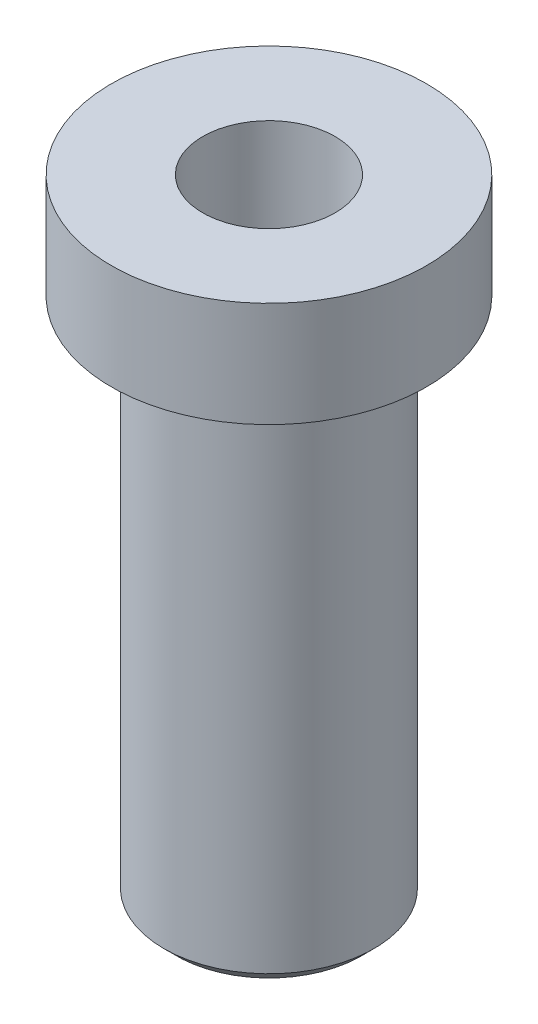
SolidWorks part; units mm, degrees
material "Plain Carbon Steel"
ref_plane "Front Plane" through (0, 0, 0) normal (0, 0, 1) x (1, 0, 0)
ref_plane "Top Plane" through (0, 0, 0) normal (0, 1, 0) x (1, 0, 0)
ref_plane "Right Plane" through (0, 0, 0) normal (1, 0, 0) x (0, 0, -1)
sketch "Pin Profile Sketch" plane through (0, 0, 0) normal (0, 0, 1) x (1, 0, 0)
  line L0 (0, 0) -> (0, 394.4019) construction
  line L2 (50, 0) -> (50, 250)
  line L3 (50, 250) -> (75, 250)
  line L4 (75, 250) -> (75, 300)
  line L7 (50, 0) -> (31.5, 0)
  line L8 (31.5, 0) -> (31.5, 300)
  line L9 (31.5, 300) -> (75, 300)
  dimension "D1" = 250
  dimension "D2" = 50
  dimension "D3" = 50
  dimension "D4" = 75
  dimension "D5" = 31.5
revolve "Pin Body Revolve" add sketch "Pin Profile Sketch" angle 360 about L0
chamfer "Shank End Chamfer 6x45°" distance 6 angle 45 1 edges at (0, 0, -50)
